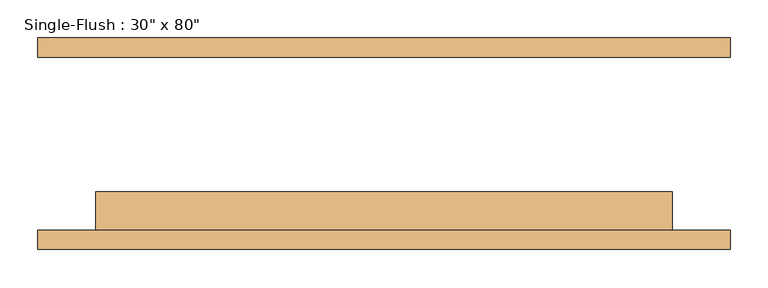
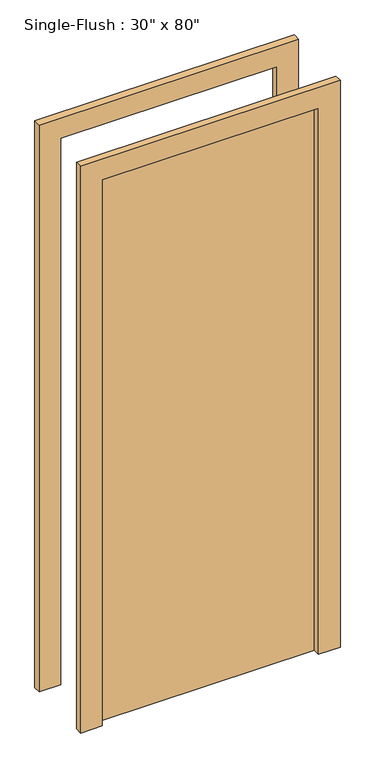
"""IFC4 building model written with IfcOpenShell, lengths in millimetres: door geometry."""

from ifc_helpers import new_model, si_unit, frame, origin, origin_with_axes, place, context, project, spatial, polyline, outline, extrude, source, transform, mapped, element, save


def door_85036156(model_context):
    return source(origin(), model_context, "Body", "SweptSolid", [
        extrude(outline(polyline([(2108.2, -457.2), (0.0, -457.2), (0.0, -381.0), (2032.0, -381.0), (2032.0, 381.0), (0.0, 381.0), (0.0, 457.2), (2108.2, 457.2), (2108.2, -457.2)])), frame((0.0, -139.7, 0.0), z_axis=(0.0, 1.0, 0.0), x_axis=(0.0, 0.0, 1.0)), (0.0, 0.0, 1.0), 25.4),
        extrude(outline(polyline([(2108.2, 457.2), (2108.2, -457.2), (0.0, -457.2), (0.0, -381.0), (2032.0, -381.0), (2032.0, 381.0), (0.0, 381.0), (0.0, 457.2), (2108.2, 457.2)])), frame((0.0, 114.3, 0.0), z_axis=(0.0, 1.0, 0.0), x_axis=(0.0, 0.0, 1.0)), (0.0, 0.0, 1.0), 25.4),
        extrude(outline(polyline([(381.0, -63.5), (381.0, -114.3), (-381.0, -114.3), (-381.0, -63.5), (381.0, -63.5)])), origin_with_axes(), (0.0, 0.0, 1.0), 2032.0),
    ])


if __name__ == "__main__":
    model = new_model("IFC4")
    model_context = context("Model", 3, world=origin())
    ifc_project = project(units=[si_unit("LENGTHUNIT", "METRE", prefix="MILLI")], contexts=[model_context])
    site = spatial("IfcSite", under=ifc_project)
    building = spatial("IfcBuilding", under=site)
    placement = place(None, origin())
    door_shape = door_85036156(model_context)
    element("IfcDoor", 1, ObjectType="Single-Flush : 30\" x 80\"", at=placement, inside=building, context=model_context, shape_type="MappedRepresentation", body=[
        mapped(door_shape, transform((0.0, 0.0, 0.0), x_axis=(1.0, 0.0, 0.0), y_axis=(0.0, 1.0, 0.0), z_axis=(0.0, 0.0, 1.0))),
    ])
    save(model, "model.ifc")

# Revit data of these elements
# Type "Single-Flush : 30\" x 80\""
#   Type Mark = "5"
#   Assembly Code = "C1020"
#   Thickness = 0' - 2"
#   Height = 6' - 8"
#   Trim Projection Ext = 0' - 1"
#   Trim Projection Int = 0' - 1"
#   Trim Width = 0' - 3"
#   Width = 2' - 6"
#   Door Material = Door - Panel
#   Frame Material = Door - Frame
#   Function = (empty or 0)
#   Wall Closure = (empty or 0)
# Element 1 (IfcDoor, "Single-Flush : 30\" x 80\"")
#   Materials on its faces: "Door - Frame", "Door - Panel"
# Materials
#   "Door - Panel": class "Wood", colour RGB 114 82 51, transparency 0
#   "Door - Frame": colour RGB 153 76 43, transparency 0
